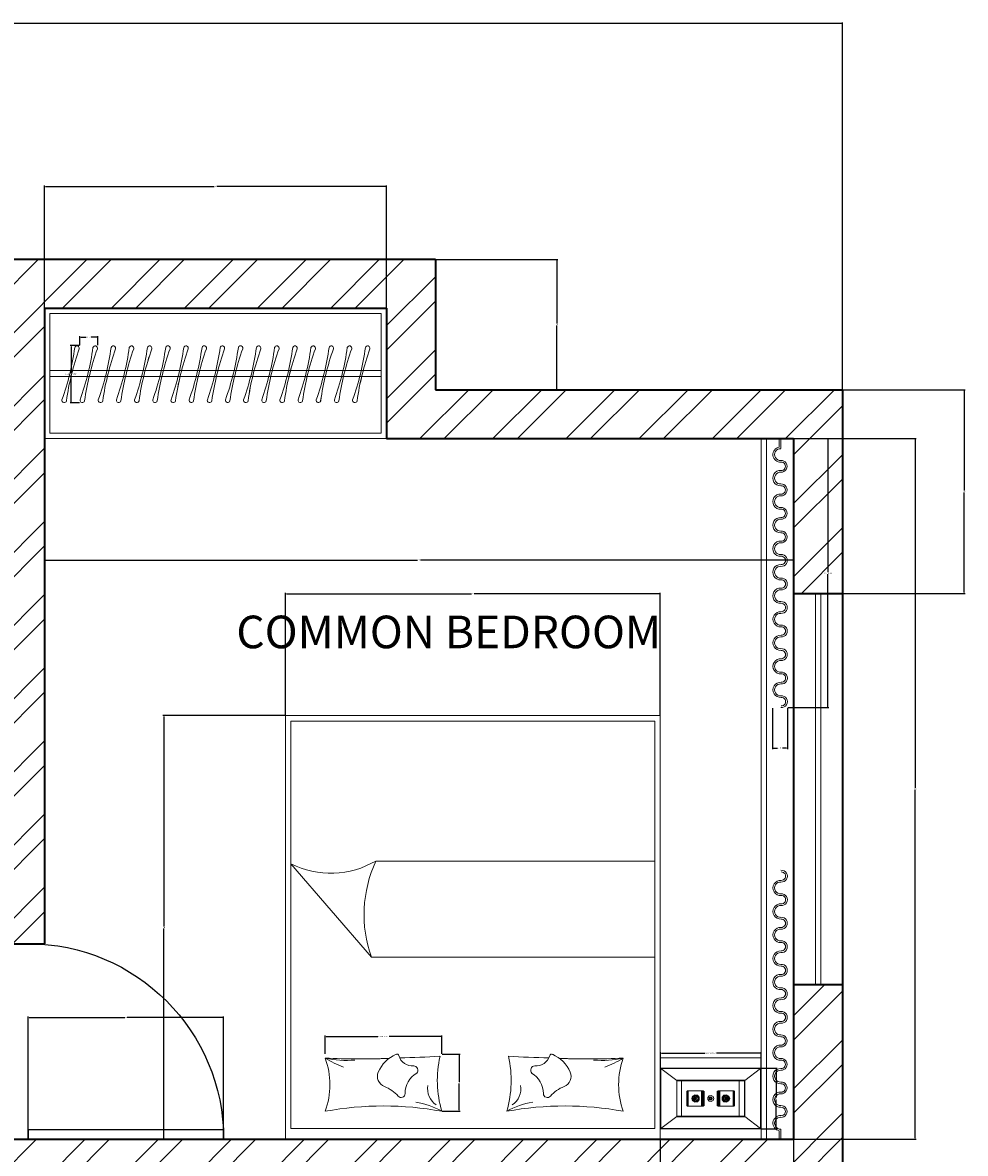
# Model space of a CAD drawing. Units: inches. Extents: x 3449 to 3843, y 1566 to 2054.
# Tile 8 of 8: x 3669 to 3843, y 1846 to 2054. Entities that reach past the tile are written whole.
import ezdxf

# ---------------------------------------------------------------- set-up
doc = ezdxf.new("R2010")
doc.units = ezdxf.units.IN
for name, color, linetype, lineweight in [('A-ANNO-DIMS', 2, 'Continuous', 18), ('A-AREA-IDEN', 7, 'Continuous', 25), ('A-DOOR', 4, 'Continuous', 25), ('A-FLOR-CASE', 7, 'Continuous', 20), ('A-FURN-DRAP', 32, 'Continuous', 13), ('A-GLAZ', 5, 'Continuous', 18), ('A-WALL', 7, 'Continuous', 35), ('A-WALL-PATT', 251, 'Continuous', 13), ('furn', 7, 'Continuous', 18)]:
    doc.layers.add(name, color=color, linetype=linetype, lineweight=lineweight)
doc.styles.get("Standard").update_dxf_attribs({"font": 'arial.ttf'})
doc.dimstyles.get("Standard").update_dxf_attribs({"dimtxt": 0.18, "dimasz": 0.18, "dimexe": 0.18, "dimexo": 0.0625, "dimgap": 0.09, "dimtad": 0, "dimtih": 1, "dimtoh": 1, "dimdec": 4, "dimzin": 0, "dimdsep": 46, "dimtxsty": 'Standard', "dimcen": 0.09, "dimadec": 0, "dimazin": 0, "dimtfac": 1, "dimtdec": 4, "dimtofl": 0, "dimtmove": 0, "dimatfit": 3, "dimfxl": 1, "dimtolj": 1, "dimtzin": 0, "dimarcsym": 0})

# ---------------------------------------------------------------- blocks, each defined once
blk = doc.blocks.new('*U5')
for p, q in [((0, 0), (0, -6)), ((36, 0), (36, -6))]:
    blk.add_line(p, q)
blk.add_lwpolyline([(0, 0), (0, 36), (1.75, 36), (1.75, 0)], close=True)
blk.add_arc((0, 0), 36, 0, 90)
blk = doc.blocks.new('12PLMP48')
for p, q in [((-4.94, 8.22), (-5, 8.31)), ((-5, 8.31), (5, 8.31)), ((-5, -8.31), (-5, 8.31)), ((-2.96, 5.62), (-4.94, 8.22)), ((4.94, 8.22), (-4.94, 8.22)), ((-4.94, 8.22), (-4.94, -8.22)), ((2.96, 5.62), (4.94, 8.22)), ((5, 8.31), (4.94, 8.22)), ((4.94, 8.22), (4.94, -8.22)), ((5, 8.31), (5, -8.31)), ((-2.94, 5.59), (-3, 5.62)), ((-3, 5.62), (3, 5.62)), ((-3, -5.63), (-3, 5.62)), ((3, 5.62), (2.94, 5.59)), ((3, -5.63), (3, 5.62)), ((2.94, 5.59), (-2.94, 5.59)), ((-2.94, 5.59), (-2.94, -5.59)), ((2.94, 4.81), (-2.94, 4.81)), ((-1.13, 3.94), (-1.25, 3.81)), ((-1.13, 3.84), (-1.25, 3.72)), ((-1.25, 3.81), (-1.25, 1.22)), ((1.13, 3.94), (-1.13, 3.94)), ((-1.13, 3.84), (-1.13, 3.94)), ((1.13, 3.84), (-1.13, 3.84)), ((1.25, 3.81), (1.13, 3.94)), ((1.13, 3.84), (1.13, 3.94)), ((1.25, 3.72), (1.13, 3.84)), ((1.25, 1.22), (1.25, 3.81)), ((2.94, -5.59), (2.94, 5.59)), ((-1.25, 3.72), (1.25, 3.72)), ((-0.62, 2.61), (-0.4, 2.98)), ((0, 2.5), (-0.62, 2.61)), ((-0.54, 2.19), (-0.62, 2.61)), ((-0.38, 2.28), (-0.54, 2.19)), ((-0.54, 2.19), (-0.21, 1.91)), ((-0.32, 2.88), (-0.49, 2.59)), ((-0.49, 2.59), (-0.43, 2.25)), ((-0.43, 2.58), (-0.28, 2.83)), ((-0.38, 2.28), (-0.43, 2.58)), ((-0.43, 2.25), (-0.17, 2.03)), ((0, 3.12), (-0.4, 2.98)), ((-0.4, 2.98), (-0.32, 2.88)), ((0, 2.5), (-0.38, 2.28)), ((-0.15, 2.09), (-0.38, 2.28)), ((0, 3), (-0.32, 2.88)), ((-0.32, 2.88), (-0.32, 2.88)), ((-0.32, 2.88), (-0.28, 2.83)), ((-0.28, 2.83), (0, 2.94)), ((-0.28, 2.83), (0, 2.5)), ((-0.21, 1.91), (0, 2.5)), ((0.21, 1.91), (-0.21, 1.91)), ((-0.17, 2.03), (0.17, 2.03)), ((0.15, 2.09), (-0.15, 2.09)), ((-0.08, 2.6), (-0.12, 2.52)), ((-0.12, 2.52), (-0.11, 2.44)), ((-0.11, 2.44), (-0.04, 2.38)), ((0, 2.62), (-0.08, 2.6)), ((-0.04, 2.38), (0.04, 2.38)), ((0, 2.5), (0, 3.12)), ((0, 3.12), (0.4, 2.98)), ((0.32, 2.88), (0, 3)), ((0, 2.94), (0.28, 2.83)), ((0, 2.5), (0.32, 2.88)), ((0.08, 2.6), (0, 2.62)), ((0.62, 2.61), (0, 2.5)), ((0.54, 2.19), (0, 2.5)), ((0, 2.5), (0.21, 1.91)), ((0.04, 2.38), (0.11, 2.44)), ((0.12, 2.52), (0.08, 2.6)), ((0.11, 2.44), (0.12, 2.52)), ((0.38, 2.28), (0.15, 2.09)), ((0.17, 2.03), (0.43, 2.25)), ((0.21, 1.91), (0.54, 2.19)), ((0.28, 2.83), (0.43, 2.58)), ((0.32, 2.88), (0.4, 2.98)), ((0.49, 2.59), (0.32, 2.88)), ((0.32, 2.88), (0.32, 2.88)), ((0.43, 2.58), (0.38, 2.28)), ((0.4, 2.98), (0.62, 2.61)), ((0.43, 2.25), (0.49, 2.59)), ((0.54, 2.19), (0.62, 2.61)), ((-1.13, 1.41), (-1.25, 1.53)), ((-1.25, 1.53), (1.25, 1.53)), ((-1.13, 1.25), (-1.25, 1.37)), ((-1.25, 1.22), (-1.13, 1.09)), ((1.13, 1.41), (-1.13, 1.41)), ((-1.13, 1.41), (-1.13, 1.09)), ((-1.13, 1.25), (1.13, 1.25)), ((-1.13, 1.09), (1.13, 1.09)), ((-0.49, -0.09), (-0.43, 0.25)), ((-0.43, 0.25), (-0.17, 0.47)), ((-0.22, 0.12), (-0.25, -0.04)), ((-0.09, 0.23), (-0.22, 0.12)), ((0.17, 0.47), (-0.17, 0.47)), ((-0.12, -0.12), (-0.12, 0.12)), ((-0.12, 0.12), (0.12, 0.12)), ((-0.09, 0.23), (0.09, 0.23)), ((0.22, 0.12), (0.09, 0.23)), ((0.12, 0.12), (0.12, -0.12)), ((0.43, 0.25), (0.17, 0.47)), ((0.25, -0.04), (0.22, 0.12)), ((0.43, 0.25), (0.49, -0.09)), ((1.25, 1.53), (1.13, 1.41)), ((1.13, 1.09), (1.13, 1.41)), ((1.13, 1.25), (1.25, 1.37)), ((1.13, 1.09), (1.25, 1.22)), ((-1.25, -1.22), (-1.13, -1.09)), ((-1.25, -1.22), (-1.25, -3.81)), ((-1.13, -1.25), (-1.25, -1.38)), ((-1.13, -1.41), (-1.25, -1.53)), ((-1.25, -1.53), (1.25, -1.53)), ((-1.13, -1.41), (-1.13, -1.09)), ((-1.13, -1.09), (1.13, -1.09)), ((1.13, -1.25), (-1.13, -1.25)), ((1.13, -1.41), (-1.13, -1.41)), ((-0.32, -0.38), (-0.49, -0.09)), ((-0.32, -0.38), (0, -0.5)), ((-0.16, -0.19), (-0.25, -0.04)), ((0, -0.25), (-0.16, -0.19)), ((0.12, -0.12), (-0.12, -0.12)), ((0.16, -0.19), (0, -0.25)), ((0.32, -0.38), (0, -0.5)), ((0.16, -0.19), (0.25, -0.04)), ((0.32, -0.38), (0.49, -0.09)), ((1.13, -1.41), (1.13, -1.09)), ((1.13, -1.09), (1.25, -1.22)), ((1.25, -1.38), (1.13, -1.25)), ((1.25, -1.53), (1.13, -1.41)), ((1.25, -3.81), (1.25, -1.22)), ((-1.13, -3.84), (-1.25, -3.72)), ((-1.25, -3.72), (1.25, -3.72)), ((-0.54, -2.19), (-0.62, -2.61)), ((0, -2.5), (-0.62, -2.61)), ((-0.62, -2.61), (-0.4, -2.98)), ((-0.21, -1.91), (-0.54, -2.19)), ((-0.54, -2.19), (0, -2.5)), ((-0.49, -2.59), (-0.43, -2.25)), ((-0.32, -2.88), (-0.49, -2.59)), ((-0.43, -2.25), (-0.17, -2.03)), ((-0.43, -2.58), (-0.38, -2.28)), ((-0.28, -2.84), (-0.43, -2.58)), ((-0.4, -2.98), (-0.32, -2.88)), ((-0.4, -2.98), (0, -3.13)), ((-0.38, -2.28), (-0.15, -2.09)), ((-0.32, -2.88), (-0.28, -2.84)), ((0, -3), (-0.32, -2.88)), ((-0.28, -2.84), (-0.08, -2.6)), ((0, -2.94), (-0.28, -2.84)), ((0.21, -1.91), (-0.21, -1.91)), ((0, -2.5), (-0.21, -1.91)), ((-0.17, -2.03), (0.17, -2.03)), ((-0.15, -2.09), (0.15, -2.09)), ((-0.11, -2.44), (-0.12, -2.52)), ((-0.12, -2.52), (-0.08, -2.6)), ((-0.04, -2.38), (-0.11, -2.44)), ((-0.08, -2.6), (0, -2.5)), ((-0.08, -2.6), (0, -2.63)), ((0.04, -2.38), (-0.04, -2.38)), ((0, -2.5), (0.21, -1.91)), ((0.11, -2.44), (0, -2.5)), ((0, -3.13), (0, -2.5)), ((0, -2.5), (0.4, -2.98)), ((0.62, -2.61), (0, -2.5)), ((0, -2.63), (0.08, -2.6)), ((0.28, -2.84), (0, -2.94)), ((0.32, -2.88), (0, -3)), ((0, -3.13), (0.4, -2.98)), ((0.11, -2.44), (0.04, -2.38)), ((0.08, -2.6), (0.12, -2.52)), ((0.38, -2.28), (0.11, -2.44)), ((0.12, -2.52), (0.11, -2.44)), ((0.15, -2.09), (0.38, -2.28)), ((0.17, -2.03), (0.43, -2.25)), ((0.21, -1.91), (0.54, -2.19)), ((0.43, -2.58), (0.28, -2.84)), ((0.49, -2.59), (0.32, -2.88)), ((0.54, -2.19), (0.38, -2.28)), ((0.38, -2.28), (0.43, -2.58)), ((0.4, -2.98), (0.62, -2.61)), ((0.43, -2.25), (0.49, -2.59)), ((0.62, -2.61), (0.54, -2.19)), ((1.25, -3.72), (1.13, -3.84)), ((-2.94, -5.59), (-3, -5.63)), ((2.94, -4.69), (-2.94, -4.69)), ((-2.94, -5.59), (2.94, -5.59)), ((-1.25, -3.81), (-1.13, -3.94)), ((-1.13, -3.94), (-1.13, -3.84)), ((1.13, -3.84), (-1.13, -3.84)), ((-1.13, -3.94), (1.13, -3.94)), ((1.13, -3.94), (1.25, -3.81)), ((1.13, -3.94), (1.13, -3.84)), ((3, -5.63), (2.94, -5.59)), ((-4.94, -8.22), (-2.96, -5.63)), ((-3, -5.63), (3, -5.63)), ((2.96, -5.63), (4.94, -8.22)), ((-4.94, -8.22), (-5, -8.31)), ((5, -8.31), (-5, -8.31)), ((4.94, -8.22), (-4.94, -8.22)), ((4.94, -8.22), (5, -8.31))]:
    blk.add_line(p, q)
blk = doc.blocks.new('PILLOW-BED')
for centre, radius, start, end in [((-58.04, 10.73), 59.02, 349.525, 10.475), ((4.89, 35.06), 14.45, 250.2291, 289.7709), ((27.88, 10.54), 21.14, 148.9025, 159.1397), ((25.99, 17.7), 16.64, 166.9326, 185.8487), ((149.01, 15.02), 139.38, 177.3527, 182.1874), ((370.18, 15.14), 360.55, 180.0403, 180.0472), ((-1.15, 12.67), 6.07, 310.2522, 339.5725), ((6.42, 9.85), 2, 66.6818, 159.5725), ((4.74, 5.96), 6.24, 23.0209, 66.6818), ((56.2, 13.08), 46.57, 181.419, 184.1998), ((10.15, 8.25), 0.362, 287.5153, 24.7447), ((3.25, 7.48), 0.73, 130.2522, 270.4936), ((3.29, 2.5), 4.25, 29.3034, 90.4936), ((10.95, 5.41), 2.59, 105.4046, 185.5925), ((370.18, 19.17), 360.55, 181.8172, 182.9967), ((-12.31, 6.94), 14.13, 330.5975, 351.1793), ((7.53, 5.25), 0.85, 231.2945, 354.0462), ((4.17, -1.03), 3.63, 80.7217, 145.7354), ((5.68, -19.42), 20.23, 77.3054, 106.2929)]:
    blk.add_arc(centre, radius, start, end)
blk = doc.blocks.new('DRAPERY-PANEL')
for p, q in [((1.19, 47.95), (1.19, 49.52)), ((1.5, 47.66), (1.5, 49.52))]:
    blk.add_line(p, q)
for centre, radius, start, end in [((1.42, 46.57), 1.4, 99.481, 274.2422), ((1.42, 46.57), 1.09, 85.7578, 274.2422), ((1.55, 44.41), 1.09, 265.7578, 94.2422), ((1.55, 44.41), 0.776, 265.7578, 94.2422), ((1.4, 42.24), 1.4, 85.7578, 274.2422), ((1.4, 42.24), 1.09, 85.7578, 274.2422), ((1.56, 40.07), 1.09, 265.7578, 94.2422), ((1.56, 40.07), 0.776, 265.7578, 94.2422), ((1.4, 37.91), 1.4, 85.7578, 274.2422), ((1.4, 37.91), 1.09, 85.7578, 274.2422), ((1.56, 35.74), 1.09, 265.7578, 94.2422), ((1.56, 35.74), 0.776, 265.7578, 94.2422), ((1.4, 33.58), 1.4, 85.7578, 274.2422), ((1.4, 33.58), 1.09, 85.7578, 274.2422), ((1.56, 31.41), 1.09, 265.7578, 94.2422), ((1.56, 31.41), 0.776, 265.7578, 94.2422), ((1.41, 29.24), 1.4, 85.7578, 274.2422), ((1.41, 29.24), 1.09, 85.7578, 274.2422), ((1.57, 27.08), 1.09, 265.7578, 94.2422), ((1.57, 27.08), 0.776, 265.7578, 94.2422), ((1.41, 24.91), 1.4, 85.7578, 274.2422), ((1.41, 24.91), 1.09, 85.7578, 274.2422), ((1.57, 22.74), 1.09, 265.7578, 94.2422), ((1.57, 22.74), 0.776, 265.7578, 94.2422), ((1.41, 20.58), 1.4, 85.7578, 274.2422), ((1.41, 20.58), 1.09, 85.7578, 274.2422), ((1.58, 18.41), 1.09, 265.7578, 94.2422), ((1.58, 18.41), 0.776, 265.7578, 94.2422), ((1.42, 16.25), 1.4, 85.7578, 274.2422), ((1.42, 16.25), 1.09, 85.7578, 274.2422), ((1.58, 14.08), 1.09, 265.7578, 94.2422), ((1.58, 14.08), 0.776, 265.7578, 94.2422), ((1.42, 11.91), 1.4, 85.7578, 274.2422), ((1.42, 11.91), 1.09, 85.7578, 274.2422), ((1.58, 9.75), 1.09, 265.7578, 94.2422), ((1.58, 9.75), 0.776, 265.7578, 94.2422), ((1.43, 7.58), 1.4, 85.7578, 274.2422), ((1.43, 7.58), 1.09, 85.7578, 274.2422), ((1.59, 5.42), 1.09, 265.7578, 94.2422), ((1.43, 3.25), 1.4, 85.7578, 274.2422), ((1.43, 3.25), 1.09, 85.7578, 274.2422), ((1.59, 5.42), 0.776, 265.7578, 94.2422), ((1.59, 1.08), 1.09, 265.7578, 94.2422), ((1.59, 1.08), 0.776, 265.7578, 94.2422)]:
    blk.add_arc(centre, radius, start, end)
blk = doc.blocks.new('WARDROBE-HANGER-A')
at = {"transparency": 33554687}
blk.add_lwpolyline([(2.38, 10.13, -1), (3.19, 9.92, 0.050016), (0.83, 0.32, -1), (0.01, 0.52, 0.050016)], format="xyb", close=True, dxfattribs=at)
blk.add_arc((49.86, -6.67), 49.53, 160.4279, 171.8811, dxfattribs=at)
blk = doc.blocks.new('WARDROBE-HANGER-B')
at = {"transparency": 33554687}
blk.add_lwpolyline([(2.37, 10.13, -1), (3.19, 9.92, 0.050016), (0.83, 0.32, -1), (0.01, 0.52, 0.050016)], format="xyb", close=True, dxfattribs=at)
blk.add_arc((49.86, -6.67), 49.53, 160.4279, 171.8811, dxfattribs=at)
blk = doc.blocks.new('GLAZING-72')
for p, q in [((0, 1), (72, 1)), ((0, 0), (72, 0))]:
    blk.add_line(p, q)
blk = doc.blocks.new('*D34')
at = {"layer": 'A-ANNO-DIMS', "color": 0, "lineweight": -2, "transparency": 16777216}
for p, q in [((3679.53, 1994.72), (3677.83, 1994.72)), ((3678.01, 1994.54), (3678.01, 1989.63)), ((3678.01, 1984.37), (3678.01, 1989.27)), ((3679.53, 1984.19), (3677.83, 1984.19))]:
    blk.add_line(p, q, dxfattribs=at)
at = {"layer": 'A-ANNO-DIMS', "color": 0, "transparency": 16777216}
for points in [[(3677.98, 1994.54), (3678.04, 1994.54), (3678.01, 1994.72)], [(3677.98, 1984.37), (3678.04, 1984.37), (3678.01, 1984.19)]]:
    blk.add_solid(points, dxfattribs=at)
at = {"layer": 'Defpoints', "color": 0, "transparency": 16777216}
for p in [(3678.01, 1994.72), (3679.59, 1994.72), (3679.59, 1984.19)]:
    blk.add_point(p, dxfattribs=at)
at = {"layer": 'A-ANNO-DIMS', "color": 0, "transparency": 16777216, "insert": (3678.01, 1989.45), "char_height": 0.18, "attachment_point": 5}
blk.add_mtext('\\A1;HANGER A 11 TYP.', dxfattribs=at)
blk = doc.blocks.new('*D35')
at = {"layer": 'A-ANNO-DIMS', "color": 0, "lineweight": -2, "transparency": 16777216}
for p, q in [((3679.59, 1994.78), (3679.59, 1996.48)), ((3679.77, 1996.3), (3680.78, 1996.3)), ((3682.71, 1996.3), (3681.7, 1996.3)), ((3682.89, 1994.78), (3682.89, 1996.48))]:
    blk.add_line(p, q, dxfattribs=at)
at = {"layer": 'A-ANNO-DIMS', "color": 0, "transparency": 16777216}
for points in [[(3679.77, 1996.33), (3679.77, 1996.27), (3679.59, 1996.3)], [(3682.71, 1996.33), (3682.71, 1996.27), (3682.89, 1996.3)]]:
    blk.add_solid(points, dxfattribs=at)
at = {"layer": 'Defpoints', "color": 0, "transparency": 16777216}
for p in [(3679.59, 1994.72), (3682.89, 1996.3), (3682.89, 1994.72)]:
    blk.add_point(p, dxfattribs=at)
at = {"layer": 'A-ANNO-DIMS', "color": 0, "transparency": 16777216, "insert": (3681.24, 1996.3), "char_height": 0.18, "attachment_point": 5}
blk.add_mtext('\\A1;3 TYP.', dxfattribs=at)
blk = doc.blocks.new('*D40')
at = {"layer": 'A-ANNO-DIMS', "color": 0, "lineweight": -2, "transparency": 16777216}
for p, q in [((3724.8, 1864.35), (3724.8, 1867.69)), ((3724.98, 1867.51), (3734.5, 1867.51)), ((3746.08, 1867.51), (3736.56, 1867.51)), ((3746.26, 1864.35), (3746.26, 1867.69))]:
    blk.add_line(p, q, dxfattribs=at)
at = {"layer": 'A-ANNO-DIMS', "color": 0, "transparency": 16777216}
for points in [[(3724.98, 1867.54), (3724.98, 1867.48), (3724.8, 1867.51)], [(3746.08, 1867.54), (3746.08, 1867.48), (3746.26, 1867.51)]]:
    blk.add_solid(points, dxfattribs=at)
at = {"layer": 'Defpoints', "color": 0, "transparency": 16777216}
for p in [(3724.8, 1867.51), (3724.8, 1864.29), (3746.26, 1864.29)]:
    blk.add_point(p, dxfattribs=at)
at = {"layer": 'A-ANNO-DIMS', "color": 0, "transparency": 16777216, "insert": (3735.53, 1867.51), "char_height": 0.18, "attachment_point": 5}
blk.add_mtext('\\A1;PILLOW 21 TYP.', dxfattribs=at)
blk = doc.blocks.new('*D41')
at = {"layer": 'A-ANNO-DIMS', "color": 0, "lineweight": -2, "transparency": 16777216}
for p, q in [((3746.32, 1864.29), (3749.66, 1864.29)), ((3749.48, 1864.11), (3749.48, 1859.21)), ((3749.48, 1853.94), (3749.48, 1858.85)), ((3746.32, 1853.76), (3749.66, 1853.76))]:
    blk.add_line(p, q, dxfattribs=at)
at = {"layer": 'A-ANNO-DIMS', "color": 0, "transparency": 16777216}
for points in [[(3749.45, 1864.11), (3749.51, 1864.11), (3749.48, 1864.29)], [(3749.45, 1853.94), (3749.51, 1853.94), (3749.48, 1853.76)]]:
    blk.add_solid(points, dxfattribs=at)
at = {"layer": 'Defpoints', "color": 0, "transparency": 16777216}
for p in [(3746.26, 1864.29), (3749.48, 1864.29), (3746.26, 1853.76)]:
    blk.add_point(p, dxfattribs=at)
at = {"layer": 'A-ANNO-DIMS', "color": 0, "transparency": 16777216, "insert": (3749.48, 1859.03), "char_height": 0.18, "attachment_point": 5}
blk.add_mtext('\\A1;11 TYP.', dxfattribs=at)
blk = doc.blocks.new('*D42')
at = {"layer": 'A-ANNO-DIMS', "color": 0, "lineweight": -2, "transparency": 16777216}
for p, q in [((3810.04, 1977.61), (3817.59, 1977.61)), ((3817.41, 1977.43), (3817.41, 1953.02)), ((3817.41, 1928.25), (3817.41, 1952.66)), ((3810.04, 1928.07), (3817.59, 1928.07))]:
    blk.add_line(p, q, dxfattribs=at)
at = {"layer": 'A-ANNO-DIMS', "color": 0, "transparency": 16777216}
for points in [[(3817.38, 1977.43), (3817.44, 1977.43), (3817.41, 1977.61)], [(3817.38, 1928.25), (3817.44, 1928.25), (3817.41, 1928.07)]]:
    blk.add_solid(points, dxfattribs=at)
at = {"layer": 'Defpoints', "color": 0, "transparency": 16777216}
for p in [(3809.98, 1977.61), (3817.41, 1977.61), (3809.98, 1928.07)]:
    blk.add_point(p, dxfattribs=at)
at = {"layer": 'A-ANNO-DIMS', "color": 0, "transparency": 16777216, "insert": (3817.41, 1952.84), "char_height": 0.18, "attachment_point": 5}
blk.add_mtext('\\A1;DRAPE 50 TYP.', dxfattribs=at)
blk = doc.blocks.new('*D43')
at = {"layer": 'A-ANNO-DIMS', "color": 0, "lineweight": -2, "transparency": 16777216}
for p, q in [((3807.18, 1928), (3807.18, 1920.45)), ((3809.98, 1928), (3809.98, 1920.45)), ((3807.36, 1920.63), (3808.12, 1920.63)), ((3809.8, 1920.63), (3809.04, 1920.63))]:
    blk.add_line(p, q, dxfattribs=at)
at = {"layer": 'A-ANNO-DIMS', "color": 0, "transparency": 16777216}
for points in [[(3807.36, 1920.66), (3807.36, 1920.6), (3807.18, 1920.63)], [(3809.8, 1920.66), (3809.8, 1920.6), (3809.98, 1920.63)]]:
    blk.add_solid(points, dxfattribs=at)
at = {"layer": 'Defpoints', "color": 0, "transparency": 16777216}
for p in [(3807.18, 1928.07), (3809.98, 1928.07), (3809.98, 1920.63)]:
    blk.add_point(p, dxfattribs=at)
at = {"layer": 'A-ANNO-DIMS', "color": 0, "transparency": 16777216, "insert": (3808.58, 1920.63), "char_height": 0.18, "attachment_point": 5}
blk.add_mtext('\\A1;3 TYP.', dxfattribs=at)
blk = doc.blocks.new('*D46')
at = {"layer": 'A-ANNO-DIMS', "color": 0, "lineweight": -2, "transparency": 16777216}
for p, q in [((3786.54, 1861.76), (3786.54, 1864.66)), ((3786.72, 1864.48), (3794.74, 1864.48)), ((3804.91, 1864.48), (3796.88, 1864.48)), ((3805.09, 1861.76), (3805.09, 1864.66))]:
    blk.add_line(p, q, dxfattribs=at)
at = {"layer": 'A-ANNO-DIMS', "color": 0, "transparency": 16777216}
for points in [[(3786.72, 1864.51), (3786.72, 1864.45), (3786.54, 1864.48)], [(3804.91, 1864.51), (3804.91, 1864.45), (3805.09, 1864.48)]]:
    blk.add_solid(points, dxfattribs=at)
at = {"layer": 'Defpoints', "color": 0, "transparency": 16777216}
for p in [(3786.54, 1864.48), (3786.54, 1861.69), (3805.09, 1861.69)]:
    blk.add_point(p, dxfattribs=at)
at = {"layer": 'A-ANNO-DIMS', "color": 0, "transparency": 16777216, "insert": (3795.81, 1864.48), "char_height": 0.18, "attachment_point": 5}
blk.add_mtext('\\A1;NIGHTSTAND 19', dxfattribs=at)
blk = doc.blocks.new('*D47')
at = {"layer": 'A-ANNO-DIMS', "color": 0, "lineweight": -2, "transparency": 16777216}
for p, q in [((3805.15, 1861.69), (3808.05, 1861.69)), ((3807.87, 1861.51), (3807.87, 1856.29)), ((3807.87, 1850.71), (3807.87, 1855.93)), ((3805.15, 1850.53), (3808.05, 1850.53))]:
    blk.add_line(p, q, dxfattribs=at)
at = {"layer": 'A-ANNO-DIMS', "color": 0, "transparency": 16777216}
for points in [[(3807.84, 1861.51), (3807.9, 1861.51), (3807.87, 1861.69)], [(3807.84, 1850.71), (3807.9, 1850.71), (3807.87, 1850.53)]]:
    blk.add_solid(points, dxfattribs=at)
at = {"layer": 'Defpoints', "color": 0, "transparency": 16777216}
for p in [(3805.09, 1861.69), (3807.87, 1861.69), (3805.09, 1850.53)]:
    blk.add_point(p, dxfattribs=at)
at = {"layer": 'A-ANNO-DIMS', "color": 0, "transparency": 16777216, "insert": (3807.87, 1856.11), "char_height": 0.18, "attachment_point": 5}
blk.add_mtext('\\A1;11', dxfattribs=at)
blk = doc.blocks.new('*D76')
at = {"layer": 'A-ANNO-DIMS', "color": 0, "lineweight": -2, "transparency": 16777216}
for p, q in [((3472.09, 2031.68), (3472.09, 2054.19)), ((3472.27, 2054.01), (3645.8, 2054.01)), ((3819.91, 2054.01), (3646.38, 2054.01)), ((3820.09, 1986.68), (3820.09, 2054.19))]:
    blk.add_line(p, q, dxfattribs=at)
at = {"layer": 'A-ANNO-DIMS', "color": 0, "transparency": 16777216}
for points in [[(3472.27, 2054.04), (3472.27, 2053.98), (3472.09, 2054.01)], [(3819.91, 2054.04), (3819.91, 2053.98), (3820.09, 2054.01)]]:
    blk.add_solid(points, dxfattribs=at)
at = {"layer": 'Defpoints', "color": 0, "transparency": 16777216}
for p in [(3820.09, 2054.01), (3472.09, 2031.61), (3820.09, 1986.61)]:
    blk.add_point(p, dxfattribs=at)
at = {"layer": 'A-ANNO-DIMS', "color": 0, "transparency": 16777216, "insert": (3646.09, 2054.01), "char_height": 0.18, "attachment_point": 5}
blk.add_mtext('\\A1;348', dxfattribs=at)
blk = doc.blocks.new('*D79')
at = {"layer": 'A-ANNO-DIMS', "color": 0, "lineweight": -2, "transparency": 16777216}
for p, q in [((3745.15, 2010.61), (3767.67, 2010.61)), ((3767.49, 2010.43), (3767.49, 1998.79)), ((3767.49, 1986.79), (3767.49, 1998.43)), ((3745.15, 1986.61), (3767.67, 1986.61))]:
    blk.add_line(p, q, dxfattribs=at)
at = {"layer": 'A-ANNO-DIMS', "color": 0, "transparency": 16777216}
for points in [[(3767.46, 2010.43), (3767.52, 2010.43), (3767.49, 2010.61)], [(3767.46, 1986.79), (3767.52, 1986.79), (3767.49, 1986.61)]]:
    blk.add_solid(points, dxfattribs=at)
at = {"layer": 'Defpoints', "color": 0, "transparency": 16777216}
for p in [(3745.09, 2010.61), (3745.09, 1986.61), (3767.49, 1986.61)]:
    blk.add_point(p, dxfattribs=at)
at = {"layer": 'A-ANNO-DIMS', "color": 0, "transparency": 16777216, "insert": (3767.49, 1998.61), "char_height": 0.18, "attachment_point": 5}
blk.add_mtext('\\A1;24', dxfattribs=at)
blk = doc.blocks.new('*D85')
at = {"layer": 'A-ANNO-DIMS', "color": 0, "lineweight": -2, "transparency": 16777216}
for p, q in [((3673.09, 1977.55), (3673.09, 1955.03)), ((3811.09, 1977.55), (3811.09, 1955.03)), ((3673.27, 1955.21), (3741.81, 1955.21)), ((3810.91, 1955.21), (3742.37, 1955.21))]:
    blk.add_line(p, q, dxfattribs=at)
at = {"layer": 'A-ANNO-DIMS', "color": 0, "transparency": 16777216}
for points in [[(3673.27, 1955.24), (3673.27, 1955.18), (3673.09, 1955.21)], [(3810.91, 1955.24), (3810.91, 1955.18), (3811.09, 1955.21)]]:
    blk.add_solid(points, dxfattribs=at)
at = {"layer": 'Defpoints', "color": 0, "transparency": 16777216}
for p in [(3673.09, 1977.61), (3811.09, 1977.61), (3673.09, 1955.21)]:
    blk.add_point(p, dxfattribs=at)
at = {"layer": 'A-ANNO-DIMS', "color": 0, "transparency": 16777216, "insert": (3742.09, 1955.21), "char_height": 0.18, "attachment_point": 5}
blk.add_mtext('\\A1;138', dxfattribs=at)
blk = doc.blocks.new('*D86')
at = {"layer": 'A-ANNO-DIMS', "color": 0, "lineweight": -2, "transparency": 16777216}
for p, q in [((3811.15, 1977.61), (3833.67, 1977.61)), ((3833.49, 1977.43), (3833.49, 1913.3)), ((3833.49, 1848.79), (3833.49, 1912.93)), ((3811.15, 1848.61), (3833.67, 1848.61))]:
    blk.add_line(p, q, dxfattribs=at)
at = {"layer": 'A-ANNO-DIMS', "color": 0, "transparency": 16777216}
for points in [[(3833.46, 1977.43), (3833.52, 1977.43), (3833.49, 1977.61)], [(3833.46, 1848.79), (3833.52, 1848.79), (3833.49, 1848.61)]]:
    blk.add_solid(points, dxfattribs=at)
at = {"layer": 'Defpoints', "color": 0, "transparency": 16777216}
for p in [(3811.09, 1977.61), (3811.09, 1848.61), (3833.49, 1848.61)]:
    blk.add_point(p, dxfattribs=at)
at = {"layer": 'A-ANNO-DIMS', "color": 0, "transparency": 16777216, "insert": (3833.49, 1913.11), "char_height": 0.18, "attachment_point": 5}
blk.add_mtext('\\A1;129', dxfattribs=at)
blk = doc.blocks.new('*D87')
at = {"layer": 'A-ANNO-DIMS', "color": 0, "lineweight": -2, "transparency": 16777216}
for p, q in [((3820.15, 1986.61), (3842.67, 1986.61)), ((3842.49, 1986.43), (3842.49, 1968.05)), ((3842.49, 1949.29), (3842.49, 1967.68)), ((3820.15, 1949.11), (3842.67, 1949.11))]:
    blk.add_line(p, q, dxfattribs=at)
at = {"layer": 'A-ANNO-DIMS', "color": 0, "transparency": 16777216}
for points in [[(3842.46, 1986.43), (3842.52, 1986.43), (3842.49, 1986.61)], [(3842.46, 1949.29), (3842.52, 1949.29), (3842.49, 1949.11)]]:
    blk.add_solid(points, dxfattribs=at)
at = {"layer": 'Defpoints', "color": 0, "transparency": 16777216}
for p in [(3820.09, 1986.61), (3820.09, 1949.11), (3842.49, 1949.11)]:
    blk.add_point(p, dxfattribs=at)
at = {"layer": 'A-ANNO-DIMS', "color": 0, "transparency": 16777216, "insert": (3842.49, 1967.86), "char_height": 0.18, "attachment_point": 5}
blk.add_mtext('\\A1;37.5', dxfattribs=at)
blk = doc.blocks.new('*D88')
at = {"layer": 'A-ANNO-DIMS', "color": 0, "lineweight": -2, "transparency": 16777216}
for p, q in [((3673.09, 2001.68), (3673.09, 2024.19)), ((3673.27, 2024.01), (3704.37, 2024.01)), ((3735.91, 2024.01), (3704.81, 2024.01)), ((3736.09, 2001.68), (3736.09, 2024.19))]:
    blk.add_line(p, q, dxfattribs=at)
at = {"layer": 'A-ANNO-DIMS', "color": 0, "transparency": 16777216}
for points in [[(3673.27, 2024.04), (3673.27, 2023.98), (3673.09, 2024.01)], [(3735.91, 2024.04), (3735.91, 2023.98), (3736.09, 2024.01)]]:
    blk.add_solid(points, dxfattribs=at)
at = {"layer": 'Defpoints', "color": 0, "transparency": 16777216}
for p in [(3736.09, 2024.01), (3673.09, 2001.61), (3736.09, 2001.61)]:
    blk.add_point(p, dxfattribs=at)
at = {"layer": 'A-ANNO-DIMS', "color": 0, "transparency": 16777216, "insert": (3704.59, 2024.01), "char_height": 0.18, "attachment_point": 5}
blk.add_mtext('\\A1;63', dxfattribs=at)
blk = doc.blocks.new('*D105')
at = {"layer": 'A-ANNO-DIMS', "color": 0, "lineweight": -2, "transparency": 16777216}
for p, q in [((3717.49, 1926.68), (3717.49, 1949.19)), ((3717.67, 1949.01), (3751.77, 1949.01)), ((3786.31, 1949.01), (3752.21, 1949.01)), ((3786.49, 1926.68), (3786.49, 1949.19))]:
    blk.add_line(p, q, dxfattribs=at)
at = {"layer": 'A-ANNO-DIMS', "color": 0, "transparency": 16777216}
for points in [[(3717.67, 1949.04), (3717.67, 1948.98), (3717.49, 1949.01)], [(3786.31, 1949.04), (3786.31, 1948.98), (3786.49, 1949.01)]]:
    blk.add_solid(points, dxfattribs=at)
at = {"layer": 'Defpoints', "color": 0, "transparency": 16777216}
for p in [(3786.49, 1949.01), (3717.49, 1926.61), (3786.49, 1926.61)]:
    blk.add_point(p, dxfattribs=at)
at = {"layer": 'A-ANNO-DIMS', "color": 0, "transparency": 16777216, "insert": (3751.99, 1949.01), "char_height": 0.18, "attachment_point": 5}
blk.add_mtext('\\A1;69', dxfattribs=at)
blk = doc.blocks.new('*D106')
at = {"layer": 'A-ANNO-DIMS', "color": 0, "lineweight": -2, "transparency": 16777216}
for p, q in [((3717.43, 1926.61), (3694.91, 1926.61)), ((3695.09, 1926.43), (3695.09, 1887.8)), ((3695.09, 1848.79), (3695.09, 1887.43)), ((3717.43, 1848.61), (3694.91, 1848.61))]:
    blk.add_line(p, q, dxfattribs=at)
at = {"layer": 'A-ANNO-DIMS', "color": 0, "transparency": 16777216}
for points in [[(3695.06, 1926.43), (3695.12, 1926.43), (3695.09, 1926.61)], [(3695.06, 1848.79), (3695.12, 1848.79), (3695.09, 1848.61)]]:
    blk.add_solid(points, dxfattribs=at)
at = {"layer": 'Defpoints', "color": 0, "transparency": 16777216}
for p in [(3695.09, 1926.61), (3717.49, 1926.61), (3717.49, 1848.61)]:
    blk.add_point(p, dxfattribs=at)
at = {"layer": 'A-ANNO-DIMS', "color": 0, "transparency": 16777216, "insert": (3695.09, 1887.61), "char_height": 0.18, "attachment_point": 5}
blk.add_mtext('\\A1;78', dxfattribs=at)
blk = doc.blocks.new('*D109')
at = {"layer": 'A-ANNO-DIMS', "color": 0, "lineweight": -2, "transparency": 16777216}
for p, q in [((3670.09, 1848.68), (3670.09, 1871.19)), ((3670.27, 1871.01), (3687.87, 1871.01)), ((3705.91, 1871.01), (3688.31, 1871.01)), ((3706.09, 1848.68), (3706.09, 1871.19))]:
    blk.add_line(p, q, dxfattribs=at)
at = {"layer": 'A-ANNO-DIMS', "color": 0, "transparency": 16777216}
for points in [[(3670.27, 1871.04), (3670.27, 1870.98), (3670.09, 1871.01)], [(3705.91, 1871.04), (3705.91, 1870.98), (3706.09, 1871.01)]]:
    blk.add_solid(points, dxfattribs=at)
at = {"layer": 'Defpoints', "color": 0, "transparency": 16777216}
for p in [(3706.09, 1871.01), (3670.09, 1848.61), (3706.09, 1848.61)]:
    blk.add_point(p, dxfattribs=at)
at = {"layer": 'A-ANNO-DIMS', "color": 0, "transparency": 16777216, "insert": (3688.09, 1871.01), "char_height": 0.18, "attachment_point": 5}
blk.add_mtext('\\A1;36', dxfattribs=at)
blk = doc.blocks.new('*D124')
at = {"layer": 'A-ANNO-DIMS', "color": 0, "lineweight": -2, "transparency": 16777216}
for p, q in [((3786.49, 1848.55), (3786.49, 1826.03)), ((3811.09, 1848.55), (3811.09, 1826.03)), ((3786.67, 1826.21), (3798.46, 1826.21)), ((3810.91, 1826.21), (3799.11, 1826.21))]:
    blk.add_line(p, q, dxfattribs=at)
at = {"layer": 'A-ANNO-DIMS', "color": 0, "transparency": 16777216}
for points in [[(3786.67, 1826.24), (3786.67, 1826.18), (3786.49, 1826.21)], [(3810.91, 1826.24), (3810.91, 1826.18), (3811.09, 1826.21)]]:
    blk.add_solid(points, dxfattribs=at)
at = {"layer": 'Defpoints', "color": 0, "transparency": 16777216}
for p in [(3786.49, 1848.61), (3811.09, 1848.61), (3786.49, 1826.21)]:
    blk.add_point(p, dxfattribs=at)
at = {"layer": 'A-ANNO-DIMS', "color": 0, "transparency": 16777216, "insert": (3798.79, 1826.21), "char_height": 0.18, "attachment_point": 5}
blk.add_mtext('\\A1;24.6', dxfattribs=at)

msp = doc.modelspace()

# ---------------------------------------------------------------- hatches: boundary and pattern name
at = {"layer": 'A-WALL-PATT'}
h = msp.add_hatch(dxfattribs=at)
h.set_pattern_fill('ANSI32', color=256)
edge = h.paths.add_edge_path()
edge.add_line((3481.088, 2022.6144), (3508.088, 2022.6144))
edge.add_line((3508.088, 2022.6144), (3508.088, 2031.6144))
edge.add_line((3508.088, 2031.6144), (3472.088, 2031.6144))
edge.add_line((3472.088, 2031.6144), (3472.088, 1779.6144))
edge.add_line((3472.088, 1779.6144), (3481.088, 1779.6144))
edge.add_line((3481.088, 1779.6144), (3481.088, 1839.6144))
edge.add_line((3481.088, 1839.6144), (3571.088, 1839.6144))
edge.add_line((3571.088, 1839.6144), (3571.088, 1824.3194))
edge.add_line((3571.088, 1824.3194), (3571.088, 1821.6144))
edge.add_line((3571.088, 1821.6144), (3580.088, 1821.6144))
edge.add_line((3580.088, 1821.6144), (3580.088, 1825.1908))
edge.add_ellipse((3580.1411, 1825.2442), major_axis=(0, 0.0754), ratio=0.99913951, start_angle=90, end_angle=135.183195, ccw=False)
edge.add_line((3580.0017, 1825.3196), (3580.0658, 1825.3196))
edge.add_line((3580.0658, 1825.3196), (3580.066, 1839.6365))
edge.add_line((3580.066, 1839.6365), (3616.088, 1839.6365))
edge.add_line((3616.088, 1839.6365), (3616.088, 1848.6144))
edge.add_line((3616.088, 1848.6144), (3610.088, 1848.6144))
edge.add_line((3610.088, 1848.6144), (3574.088, 1848.6144))
edge.add_line((3574.088, 1848.6144), (3481.088, 1848.6144))
edge.add_line((3481.088, 1848.6144), (3481.088, 1872.6144))
edge.add_line((3481.088, 1872.6144), (3481.088, 2022.6144))
h.paths.add_polyline_path([(3550.088, 1779.6144), (3616.088, 1779.6144), (3616.088, 1791.6144), (3505.088, 1791.6144), (3505.088, 1779.6144), (3541.088, 1779.6144), (3541.088, 1657.6144), (3481.088, 1657.6144), (3481.088, 1588.6144), (3496.088, 1588.6144), (3496.088, 1594.6144), (3496.088, 1597.6144), (3490.088, 1597.6144), (3490.088, 1648.6144), (3550.088, 1648.6144)])
h.paths.add_polyline_path([(3775.088, 1612.6144), (3766.088, 1612.6144), (3766.088, 1597.6144), (3536.088, 1597.6144), (3536.088, 1588.6144), (3775.088, 1588.6144)])
h.paths.add_polyline_path([(3820.088, 1756.6144), (3811.088, 1756.6144), (3811.088, 1732.6144), (3664.088, 1732.6144), (3664.088, 1723.6144), (3766.088, 1723.6144), (3766.088, 1708.6144), (3775.088, 1708.6144), (3775.088, 1723.6144), (3820.088, 1723.6144)])
h.paths.add_polyline_path([(3820.088, 1986.6144), (3745.088, 1986.6144), (3745.088, 2010.6144), (3664.088, 2010.6144), (3664.088, 1992.6144), (3652.088, 1992.6144), (3652.088, 1983.6144), (3664.088, 1983.6144), (3664.088, 1893.6144), (3648.793, 1893.6144), (3607.088, 1893.6144), (3607.088, 1884.6144), (3673.088, 1884.6144), (3673.088, 2001.6144), (3736.088, 2001.6144), (3736.088, 1977.6144), (3811.088, 1977.6144), (3811.088, 1949.1144), (3820.088, 1949.1144)])
h.paths.add_polyline_path([(3628.088, 1992.6144), (3616.088, 1992.6144), (3616.088, 2031.6144), (3580.088, 2031.6144), (3580.088, 2022.6144), (3607.088, 2022.6144), (3607.088, 1921.6144), (3613.088, 1921.6144), (3616.088, 1921.6144), (3616.088, 1983.6144), (3628.088, 1983.6144)])
h.paths.add_polyline_path([(3820.088, 1877.1144), (3811.088, 1877.1144), (3811.088, 1848.6144), (3664.088, 1848.6144), (3664.088, 1839.6144), (3700.088, 1839.6144), (3811.088, 1839.6144), (3811.088, 1815.6144), (3820.088, 1815.6144)])

# ---------------------------------------------------------------- linework, layer by layer
at = {"layer": 'A-FLOR-CASE'}
msp.add_line((3735.088, 1990.1595), (3735.088, 1989.0693), dxfattribs=at)
for points in [[(3736.088, 1977.6144), (3673.088, 1977.6144), (3673.088, 2001.6144), (3736.088, 2001.6144)], [(3735.088, 1978.6144), (3674.088, 1978.6144), (3674.088, 2000.6144), (3735.088, 2000.6144)], [(3674.088, 1990.1595), (3735.088, 1990.1595)], [(3674.088, 1989.0693), (3735.088, 1989.0693)]]:
    msp.add_lwpolyline(points, close=True, dxfattribs=at)
at = {"layer": 'A-FURN-DRAP'}
for p, q in [((3805.088, 1977.6144), (3805.088, 1848.6144)), ((3806.088, 1977.6144), (3806.088, 1848.6144))]:
    msp.add_line(p, q, dxfattribs=at)
at = {"layer": 'A-WALL'}
for p, q in [((3616.088, 2010.6144), (3745.088, 2010.6144)), ((3664.088, 2010.6144), (3745.088, 2010.6144)), ((3745.088, 2010.6144), (3745.088, 1986.6144)), ((3673.088, 2001.6144), (3673.088, 1884.6144)), ((3673.088, 2001.6144), (3736.088, 2001.6144)), ((3736.088, 2001.6144), (3736.088, 1977.6144)), ((3745.088, 1986.6144), (3820.088, 1986.6144)), ((3820.088, 1986.6144), (3820.088, 1949.1144)), ((3736.088, 1977.6144), (3811.088, 1977.6144)), ((3811.088, 1977.6144), (3811.088, 1848.6144)), ((3811.088, 1949.1144), (3820.088, 1949.1144)), ((3820.088, 1949.1144), (3820.088, 1756.6144)), ((3607.088, 1884.6144), (3673.088, 1884.6144)), ((3811.088, 1877.1144), (3820.088, 1877.1144)), ((3664.088, 1848.6144), (3811.088, 1848.6144))]:
    msp.add_line(p, q, dxfattribs=at)
at = {"layer": 'furn'}
for p, q in [((3733.2968, 1882.1177), (3718.488, 1899.2947)), ((3734.1334, 1899.8382), (3785.488, 1899.8382)), ((3785.488, 1882.1177), (3733.2968, 1882.1177))]:
    msp.add_line(p, q, dxfattribs=at)
for points in [[(3717.488, 1926.6144), (3786.488, 1926.6144), (3786.488, 1848.6144), (3717.488, 1848.6144)], [(3718.488, 1925.6144), (3785.488, 1925.6144), (3785.488, 1850.6144), (3718.488, 1850.6144)], [(3786.488, 1863.6144), (3805.088, 1863.6144), (3805.088, 1848.6144), (3786.488, 1848.6144)]]:
    msp.add_lwpolyline(points, close=True, dxfattribs=at)
for centre, radius, start, end in [((3725.8002, 1914.2618), 16.6578, 243.962328, 300.017373), ((3755.4326, 1889.9526), 23.4815, 155.102404, 199.491316)]:
    msp.add_arc(centre, radius, start, end, dxfattribs=at)

# ---------------------------------------------------------------- block references
at = {"layer": 'A-DOOR', "xscale": -1, "rotation": 270}
msp.add_blockref('*U5', (3670.088, 1848.6144), dxfattribs=at)
at = {"layer": 'A-FLOR-CASE'}
for name, p in [('WARDROBE-HANGER-B', (3676.2967, 1984.23)), ('WARDROBE-HANGER-A', (3679.6372, 1984.23)), ('WARDROBE-HANGER-B', (3682.9912, 1984.23)), ('WARDROBE-HANGER-A', (3686.3318, 1984.23)), ('WARDROBE-HANGER-A', (3689.6722, 1984.23)), ('WARDROBE-HANGER-A', (3693.0264, 1984.23)), ('WARDROBE-HANGER-B', (3696.3804, 1984.23)), ('WARDROBE-HANGER-A', (3699.721, 1984.23)), ('WARDROBE-HANGER-B', (3703.075, 1984.23)), ('WARDROBE-HANGER-A', (3706.4156, 1984.23)), ('WARDROBE-HANGER-A', (3709.7559, 1984.23)), ('WARDROBE-HANGER-A', (3713.0963, 1984.23)), ('WARDROBE-HANGER-B', (3716.4503, 1984.23)), ('WARDROBE-HANGER-A', (3719.7909, 1984.23)), ('WARDROBE-HANGER-A', (3723.1313, 1984.23)), ('WARDROBE-HANGER-A', (3726.4855, 1984.23)), ('WARDROBE-HANGER-B', (3729.8395, 1984.23))]:
    msp.add_blockref(name, p, dxfattribs=at)
at = {"layer": 'A-FURN-DRAP'}
msp.add_blockref('DRAPERY-PANEL', (3807.247, 1928.096), dxfattribs=at)
at = {"layer": 'A-FURN-DRAP', "extrusion": (0, 0, -1), "zscale": -1, "rotation": 180}
msp.add_blockref('DRAPERY-PANEL', (-3807.247, 1898.1328), dxfattribs=at)
at = {"layer": 'A-GLAZ', "rotation": 89.99999999999856}
msp.add_blockref('GLAZING-72', (3816.0884, 1877.1144), dxfattribs=at)
at = {"layer": 'furn', "rotation": 89.99999999999952}
msp.add_blockref('PILLOW-BED', (3746.2604, 1853.7639), dxfattribs=at)
at = {"layer": 'furn', "extrusion": (0, 0, -1), "zscale": -1, "rotation": 89.99999999999982}
msp.add_blockref('PILLOW-BED', (-3758.2432, 1853.7639), dxfattribs=at)
at = {"layer": 'furn', "xscale": 1.115911277925004, "yscale": 1.115911277925004, "zscale": 1.115911277925004, "rotation": 90}
msp.add_blockref('12PLMP48', (3795.8109, 1856.1144), dxfattribs=at)

# ---------------------------------------------------------------- texts
at = {"layer": 'A-AREA-IDEN', "insert": (3708.4257, 1945.0108), "char_height": 6, "attachment_point": 1}
msp.add_mtext_dynamic_manual_height_columns('COMMON BEDROOM', width=95.638287, gutter_width=12.5, heights=[0], dxfattribs=at)

# ---------------------------------------------------------------- dimensions: what is measured, and where the dimension line sits
at = {"layer": 'A-ANNO-DIMS'}
for base, p1, p2, picture, middle in [((3820.088, 2054.0144), (3472.088, 2031.6144), (3820.088, 1986.6144), '*D76', (3646.088, 2054.0144)), ((3736.088, 2024.0144), (3673.088, 2001.6144), (3736.088, 2001.6144), '*D88', (3704.588, 2024.0144)), ((3786.488, 1949.0144), (3717.488, 1926.6144), (3786.488, 1926.6144), '*D105', (3751.988, 1949.0144)), ((3706.088, 1871.0144), (3670.088, 1848.6144), (3706.088, 1848.6144), '*D109', (3688.088, 1871.0144))]:
    dim = msp.add_linear_dim(base=base, p1=p1, p2=p2, dimstyle='Standard', override={"dimdec": 0, "dimlfac": 1, "dimrnd": 0, "dimzin": 0, "dimdsep": 46, "dimlunit": 2}, dxfattribs=at)
    dim.commit()
    dim.dimension.update_dxf_attribs({"geometry": picture, "text_midpoint": middle})
for base, p1, p2, angle, override, picture, middle in [((3767.488, 1986.6144), (3745.088, 2010.6144), (3745.088, 1986.6144), 270, {"dimdec": 0, "dimlfac": 1, "dimrnd": 0, "dimzin": 0, "dimdsep": 46, "dimlunit": 2}, '*D79', (3767.488, 1998.6144)), ((3842.488, 1949.1144), (3820.088, 1986.6144), (3820.088, 1949.1144), 270, {"dimdec": 1, "dimlfac": 1, "dimrnd": 0, "dimzin": 0, "dimdsep": 46, "dimlunit": 2}, '*D87', (3842.488, 1967.8644)), ((3673.088, 1955.2144), (3811.088, 1977.6144), (3673.088, 1977.6144), 180, {"dimdec": 0, "dimlfac": 1, "dimrnd": 0, "dimzin": 0, "dimdsep": 46, "dimlunit": 2}, '*D85', (3742.088, 1955.2144)), ((3833.488, 1848.6144), (3811.088, 1977.6144), (3811.088, 1848.6144), 270, {"dimdec": 0, "dimlfac": 1, "dimrnd": 0, "dimzin": 0, "dimdsep": 46, "dimlunit": 2}, '*D86', (3833.488, 1913.1144)), ((3695.088, 1926.6144), (3717.488, 1848.6144), (3717.488, 1926.6144), 90, {"dimdec": 0, "dimlfac": 1, "dimrnd": 0, "dimzin": 0, "dimdsep": 46, "dimlunit": 2}, '*D106', (3695.088, 1887.6144)), ((3807.871, 1861.6939), (3805.088, 1850.5349), (3805.088, 1861.6939), 90, {"dimdec": 0, "dimlfac": 1, "dimrnd": 0, "dimzin": 0, "dimdsep": 46, "dimlunit": 2}, '*D47', (3807.871, 1856.1144)), ((3786.488, 1826.2144), (3811.088, 1848.6144), (3786.488, 1848.6144), 180, {"dimdec": 1, "dimlfac": 1, "dimrnd": 0, "dimzin": 0, "dimdsep": 46, "dimlunit": 2}, '*D124', (3798.788, 1826.2144))]:
    dim = msp.add_linear_dim(base=base, p1=p1, p2=p2, angle=angle, dimstyle='Standard', override=override, dxfattribs=at)
    dim.commit()
    dim.dimension.update_dxf_attribs({"geometry": picture, "text_midpoint": middle})
for base, p1, p2, picture, middle in [((3682.8894, 1996.2972), (3679.5932, 1994.7174), (3682.8894, 1994.7174), '*D35', (3681.2413, 1996.2972)), ((3809.9764, 1920.6343), (3807.1789, 1928.0665), (3809.9764, 1928.0665), '*D43', (3808.5777, 1920.6343))]:
    dim = msp.add_linear_dim(base=base, p1=p1, p2=p2, text='<> TYP.', dimstyle='Standard', override={"dimdec": 0, "dimlfac": 1, "dimrnd": 0, "dimzin": 0, "dimdsep": 46, "dimlunit": 2}, dxfattribs=at)
    dim.commit()
    dim.dimension.update_dxf_attribs({"geometry": picture, "text_midpoint": middle})
for base, p1, p2, angle, text, picture, middle in [((3678.0134, 1994.7174), (3679.5932, 1984.1858), (3679.5932, 1994.7174), 90, 'HANGER A <> TYP.', '*D34', (3678.0134, 1989.4516)), ((3817.4086, 1977.6144), (3809.9764, 1928.0665), (3809.9764, 1977.6144), 90, 'DRAPE <> TYP.', '*D42', (3817.4086, 1952.8404)), ((3724.7994, 1867.5073), (3746.2604, 1864.2882), (3724.7994, 1864.2882), 180, 'PILLOW <> TYP.', '*D40', (3735.5299, 1867.5073)), ((3749.4796, 1864.2882), (3746.2604, 1853.7635), (3746.2604, 1864.2882), 90, '<> TYP.', '*D41', (3749.4796, 1859.0258)), ((3786.5351, 1864.4768), (3805.088, 1861.6939), (3786.5351, 1861.6939), 180, 'NIGHTSTAND <>', '*D46', (3795.8115, 1864.4768))]:
    dim = msp.add_linear_dim(base=base, p1=p1, p2=p2, angle=angle, text=text, dimstyle='Standard', override={"dimdec": 0, "dimlfac": 1, "dimrnd": 0, "dimzin": 0, "dimdsep": 46, "dimlunit": 2}, dxfattribs=at)
    dim.commit()
    dim.dimension.update_dxf_attribs({"geometry": picture, "text_midpoint": middle})

doc.saveas('drawing.dxf')
